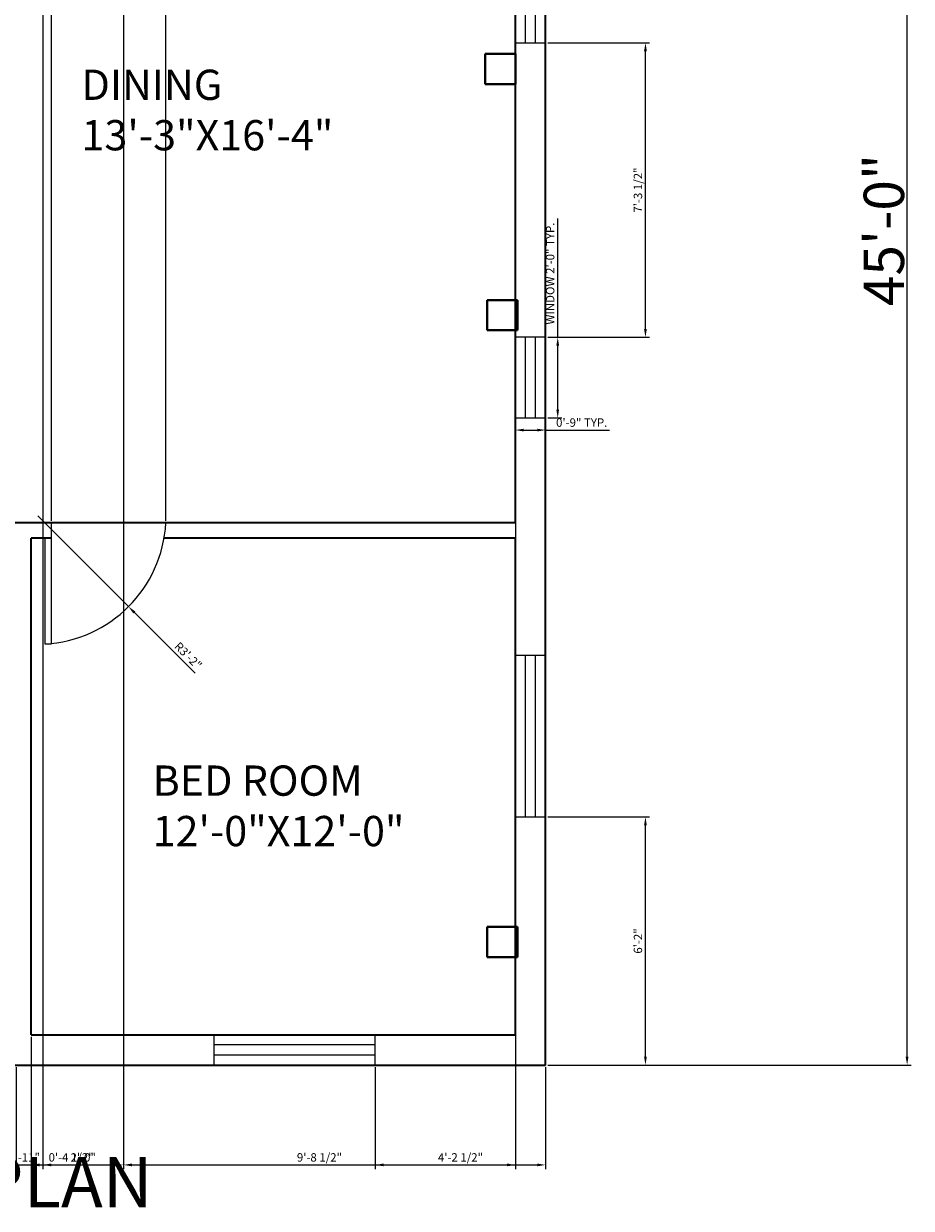
# Model space of a CAD drawing. Units: millimetres. Extents: x 2124 to 2653, y 1244 to 1836.
# Tile 2 of 4: x 2389 to 2653, y 1244 to 1597. Entities that reach past the tile are written whole.
import ezdxf

# ---------------------------------------------------------------- set-up
doc = ezdxf.new("R2010")
doc.units = ezdxf.units.MM
for name, color, linetype, lineweight in [('A-ANNO-DIMS', 2, 'Continuous', 18), ('A-ANNO-TITL', 7, 'Continuous', 35), ('A-AREA-IDEN', 7, 'Continuous', 18), ('A-COLS', 1, 'Continuous', 40), ('A-DOOR', 3, 'Continuous', 18), ('A-GLAZ', 4, 'Continuous', 18), ('A-WALL', 7, 'Continuous', 35)]:
    doc.layers.add(name, color=color, linetype=linetype, lineweight=lineweight)
doc.styles.get("Standard").update_dxf_attribs({"font": 'arial.ttf'})
doc.dimstyles.new('ISO-25', dxfattribs={"dimtxt": 2.5, "dimasz": 2.5, "dimexe": 1.25, "dimexo": 0.625, "dimtad": 1, "dimdec": 0, "dimlunit": 3, "dimtxsty": 'Standard', "dimcen": 2.5, "dimadec": 0, "dimazin": 0, "dimtfac": 1, "dimtdec": 0, "dimtmove": 0, "dimatfit": 3, "dimfxl": 1, "dimarcsym": 0})

# ---------------------------------------------------------------- blocks, each defined once
blk = doc.blocks.new('*D9')
at = {"layer": 'A-ANNO-DIMS', "color": 0, "lineweight": -2, "transparency": 16777216}
for p, q in [((2544.38, 1783.74), (2652.54, 1783.74)), ((2651.29, 1289.47), (2651.29, 1781.24)), ((2544.38, 1286.97), (2652.54, 1286.97))]:
    blk.add_line(p, q, dxfattribs=at)
at = {"layer": 'A-ANNO-DIMS', "color": 0, "transparency": 16777216}
for points in [[(2650.87, 1781.24), (2651.71, 1781.24), (2651.29, 1783.74)], [(2650.87, 1289.47), (2651.71, 1289.47), (2651.29, 1286.97)]]:
    blk.add_solid(points, dxfattribs=at)
at = {"layer": 'Defpoints', "color": 0, "transparency": 16777216}
for p in [(2543.76, 1783.74), (2651.29, 1783.74), (2543.76, 1286.97)]:
    blk.add_point(p, dxfattribs=at)
at = {"layer": 'A-ANNO-DIMS', "color": 0, "transparency": 16777216, "insert": (2644.38, 1535.36), "char_height": 2.5, "width": 21.1968, "attachment_point": 5, "rotation": 90}
blk.add_mtext('{\\fCambria|b0|i0|c0|p18;\\H4.8x;45\'-0"}', dxfattribs=at)
blk = doc.blocks.new('WINDOW-4FT')
for p, q in [((48, 9), (0, 9)), ((0, 9), (0, 0)), ((48, 0), (48, 9)), ((48, 6), (0, 6)), ((48, 3), (0, 3)), ((0, 0), (48, 0))]:
    blk.add_line(p, q)
blk = doc.blocks.new('WINDOW-2FT')
for p, q in [((9, 24), (0, 24)), ((0, 24), (0, 0)), ((3, 0), (3, 24)), ((6, 0), (6, 24)), ((9, 0), (9, 24)), ((0, 0), (9, 0))]:
    blk.add_line(p, q)
blk = doc.blocks.new('COLUMN-9IN-SQ')
for p, q in [((9, 9), (0, 9)), ((0, 9), (0, 0)), ((9, 0), (9, 9)), ((0, 0), (9, 0))]:
    blk.add_line(p, q)
blk = doc.blocks.new('*D18')
at = {"layer": 'A-ANNO-DIMS', "color": 0, "lineweight": -2, "transparency": 16777216}
for p, q in [((2547.36, 1503.47), (2547.36, 1538.85)), ((2544.38, 1503.47), (2548.61, 1503.47)), ((2547.36, 1481.97), (2547.36, 1500.97)), ((2544.38, 1479.47), (2548.61, 1479.47))]:
    blk.add_line(p, q, dxfattribs=at)
at = {"layer": 'A-ANNO-DIMS', "color": 0, "transparency": 16777216}
for points in [[(2546.94, 1500.97), (2547.77, 1500.97), (2547.36, 1503.47)], [(2546.94, 1481.97), (2547.77, 1481.97), (2547.36, 1479.47)]]:
    blk.add_solid(points, dxfattribs=at)
at = {"layer": 'Defpoints', "color": 0, "transparency": 16777216}
for p in [(2543.76, 1503.47), (2547.36, 1503.47), (2543.76, 1479.47)]:
    blk.add_point(p, dxfattribs=at)
at = {"layer": 'A-ANNO-DIMS', "color": 0, "transparency": 16777216, "insert": (2545.44, 1522.41), "char_height": 2.5, "attachment_point": 5, "rotation": 90}
blk.add_mtext('WINDOW 2\'-0" TYP.', dxfattribs=at)
blk = doc.blocks.new('*D19')
at = {"layer": 'A-ANNO-DIMS', "color": 0, "lineweight": -2, "transparency": 16777216}
for p, q in [((2534.76, 1478.84), (2534.76, 1474.62)), ((2543.76, 1478.84), (2543.76, 1474.62)), ((2537.26, 1475.87), (2541.26, 1475.87)), ((2543.76, 1475.87), (2562.75, 1475.87))]:
    blk.add_line(p, q, dxfattribs=at)
at = {"layer": 'A-ANNO-DIMS', "color": 0, "transparency": 16777216}
for points in [[(2537.26, 1476.28), (2537.26, 1475.45), (2534.76, 1475.87)], [(2541.26, 1476.28), (2541.26, 1475.45), (2543.76, 1475.87)]]:
    blk.add_solid(points, dxfattribs=at)
at = {"layer": 'Defpoints', "color": 0, "transparency": 16777216}
for p in [(2534.76, 1479.47), (2543.76, 1479.47), (2543.76, 1475.87)]:
    blk.add_point(p, dxfattribs=at)
at = {"layer": 'A-ANNO-DIMS', "color": 0, "transparency": 16777216, "insert": (2554.5, 1477.77), "char_height": 2.5, "attachment_point": 5}
blk.add_mtext('0\'-9" TYP.', dxfattribs=at)
blk = doc.blocks.new('*D23')
at = {"layer": 'A-ANNO-DIMS', "color": 0, "lineweight": -2, "transparency": 16777216}
for p, q in [((2493.1, 1286.35), (2493.1, 1256.02)), ((2543.76, 1286.35), (2543.76, 1256.02)), ((2495.6, 1257.27), (2541.26, 1257.27))]:
    blk.add_line(p, q, dxfattribs=at)
at = {"layer": 'A-ANNO-DIMS', "color": 0, "transparency": 16777216}
for points in [[(2495.6, 1257.69), (2495.6, 1256.86), (2493.1, 1257.27)], [(2541.26, 1257.69), (2541.26, 1256.86), (2543.76, 1257.27)]]:
    blk.add_solid(points, dxfattribs=at)
at = {"layer": 'Defpoints', "color": 0, "transparency": 16777216}
for p in [(2493.1, 1286.97), (2543.76, 1286.97), (2543.76, 1257.27)]:
    blk.add_point(p, dxfattribs=at)
at = {"layer": 'A-ANNO-DIMS', "color": 0, "transparency": 16777216, "insert": (2518.43, 1259.19), "char_height": 2.5, "attachment_point": 5}
blk.add_mtext('4\'-2 1/2"', dxfattribs=at)
blk = doc.blocks.new('*D26')
at = {"layer": 'A-ANNO-DIMS', "color": 0, "lineweight": -2, "transparency": 16777216}
for p, q in [((2544.38, 1591.07), (2574.71, 1591.07)), ((2573.46, 1505.97), (2573.46, 1588.57)), ((2544.38, 1503.47), (2574.71, 1503.47))]:
    blk.add_line(p, q, dxfattribs=at)
at = {"layer": 'A-ANNO-DIMS', "color": 0, "transparency": 16777216}
for points in [[(2573.04, 1588.57), (2573.87, 1588.57), (2573.46, 1591.07)], [(2573.04, 1505.97), (2573.87, 1505.97), (2573.46, 1503.47)]]:
    blk.add_solid(points, dxfattribs=at)
at = {"layer": 'Defpoints', "color": 0, "transparency": 16777216}
for p in [(2543.76, 1591.07), (2573.46, 1591.07), (2543.76, 1503.47)]:
    blk.add_point(p, dxfattribs=at)
at = {"layer": 'A-ANNO-DIMS', "color": 0, "transparency": 16777216, "insert": (2571.54, 1547.27), "char_height": 2.5, "attachment_point": 5, "rotation": 90}
blk.add_mtext('7\'-3 1/2"', dxfattribs=at)
blk = doc.blocks.new('*D27')
at = {"layer": 'A-ANNO-DIMS', "color": 0, "lineweight": -2, "transparency": 16777216}
for p, q in [((2544.38, 1360.81), (2574.71, 1360.81)), ((2573.46, 1289.47), (2573.46, 1358.31)), ((2544.38, 1286.97), (2574.71, 1286.97))]:
    blk.add_line(p, q, dxfattribs=at)
at = {"layer": 'A-ANNO-DIMS', "color": 0, "transparency": 16777216}
for points in [[(2573.04, 1358.31), (2573.87, 1358.31), (2573.46, 1360.81)], [(2573.04, 1289.47), (2573.87, 1289.47), (2573.46, 1286.97)]]:
    blk.add_solid(points, dxfattribs=at)
at = {"layer": 'Defpoints', "color": 0, "transparency": 16777216}
for p in [(2543.76, 1360.81), (2573.46, 1360.81), (2543.76, 1286.97)]:
    blk.add_point(p, dxfattribs=at)
at = {"layer": 'A-ANNO-DIMS', "color": 0, "transparency": 16777216, "insert": (2571.55, 1323.89), "char_height": 2.5, "attachment_point": 5, "rotation": 90}
blk.add_mtext('6\'-2"', dxfattribs=at)
blk = doc.blocks.new('*D43')
at = {"layer": 'A-ANNO-DIMS', "color": 0, "lineweight": -2, "transparency": 16777216}
for p, q in [((2383.02, 1645.62), (2383.02, 1256.02)), ((2394.21, 1645.62), (2394.21, 1256.02)), ((2385.52, 1257.27), (2391.71, 1257.27))]:
    blk.add_line(p, q, dxfattribs=at)
at = {"layer": 'A-ANNO-DIMS', "color": 0, "transparency": 16777216}
for points in [[(2385.52, 1257.69), (2385.52, 1256.86), (2383.02, 1257.27)], [(2391.71, 1257.69), (2391.71, 1256.86), (2394.21, 1257.27)]]:
    blk.add_solid(points, dxfattribs=at)
at = {"layer": 'Defpoints', "color": 0, "transparency": 16777216}
for p in [(2383.02, 1646.24), (2394.21, 1646.24), (2394.21, 1257.27)]:
    blk.add_point(p, dxfattribs=at)
at = {"layer": 'A-ANNO-DIMS', "color": 0, "transparency": 16777216, "insert": (2388.62, 1259.18), "char_height": 2.5, "attachment_point": 5}
blk.add_mtext('0\'-11"', dxfattribs=at)
blk = doc.blocks.new('*D44')
at = {"layer": 'A-ANNO-DIMS', "color": 0, "lineweight": -2, "transparency": 16777216}
for p, q in [((2394.21, 1645.62), (2394.21, 1256.02)), ((2418.21, 1645.62), (2418.21, 1256.02)), ((2396.71, 1257.27), (2415.71, 1257.27))]:
    blk.add_line(p, q, dxfattribs=at)
at = {"layer": 'A-ANNO-DIMS', "color": 0, "transparency": 16777216}
for points in [[(2396.71, 1257.69), (2396.71, 1256.86), (2394.21, 1257.27)], [(2415.71, 1257.69), (2415.71, 1256.86), (2418.21, 1257.27)]]:
    blk.add_solid(points, dxfattribs=at)
at = {"layer": 'Defpoints', "color": 0, "transparency": 16777216}
for p in [(2394.21, 1646.24), (2418.21, 1646.24), (2418.21, 1257.27)]:
    blk.add_point(p, dxfattribs=at)
at = {"layer": 'A-ANNO-DIMS', "color": 0, "transparency": 16777216, "insert": (2406.21, 1259.18), "char_height": 2.5, "attachment_point": 5}
blk.add_mtext('2\'-0"', dxfattribs=at)
blk = doc.blocks.new('*D45')
at = {"layer": 'A-ANNO-DIMS', "color": 0, "lineweight": -2, "transparency": 16777216}
for p, q in [((2418.21, 1645.62), (2418.21, 1256.02)), ((2534.76, 1645.62), (2534.76, 1256.02)), ((2420.71, 1257.27), (2532.26, 1257.27))]:
    blk.add_line(p, q, dxfattribs=at)
at = {"layer": 'A-ANNO-DIMS', "color": 0, "transparency": 16777216}
for points in [[(2420.71, 1257.69), (2420.71, 1256.86), (2418.21, 1257.27)], [(2532.26, 1257.69), (2532.26, 1256.86), (2534.76, 1257.27)]]:
    blk.add_solid(points, dxfattribs=at)
at = {"layer": 'Defpoints', "color": 0, "transparency": 16777216}
for p in [(2418.21, 1646.24), (2534.76, 1646.24), (2534.76, 1257.27)]:
    blk.add_point(p, dxfattribs=at)
at = {"layer": 'A-ANNO-DIMS', "color": 0, "transparency": 16777216, "insert": (2476.48, 1259.19), "char_height": 2.5, "attachment_point": 5}
blk.add_mtext('9\'-8 1/2"', dxfattribs=at)
blk = doc.blocks.new('*D47')
at = {"layer": 'A-ANNO-DIMS', "color": 0, "lineweight": -2, "transparency": 16777216}
for p, q in [((2365.24, 1448.87), (2365.24, 1814.69)), ((2367.74, 1813.44), (2394.29, 1813.44)), ((2396.79, 1448.87), (2396.79, 1814.69))]:
    blk.add_line(p, q, dxfattribs=at)
at = {"layer": 'A-ANNO-DIMS', "color": 0, "transparency": 16777216}
for points in [[(2367.74, 1813.86), (2367.74, 1813.02), (2365.24, 1813.44)], [(2394.29, 1813.86), (2394.29, 1813.02), (2396.79, 1813.44)]]:
    blk.add_solid(points, dxfattribs=at)
at = {"layer": 'Defpoints', "color": 0, "transparency": 16777216}
for p in [(2396.79, 1813.44), (2365.24, 1448.24), (2396.79, 1448.24)]:
    blk.add_point(p, dxfattribs=at)
at = {"layer": 'A-ANNO-DIMS', "color": 0, "transparency": 16777216, "insert": (2381.02, 1815.36), "char_height": 2.5, "attachment_point": 5}
blk.add_mtext('2\'-7 1/2"', dxfattribs=at)
blk = doc.blocks.new('*D48')
at = {"layer": 'A-ANNO-DIMS', "color": 0, "lineweight": -2, "transparency": 16777216}
for p, q in [((2396.79, 1448.87), (2396.79, 1814.69)), ((2399.29, 1813.44), (2428.29, 1813.44)), ((2430.79, 1448.87), (2430.79, 1814.69))]:
    blk.add_line(p, q, dxfattribs=at)
at = {"layer": 'A-ANNO-DIMS', "color": 0, "transparency": 16777216}
for points in [[(2399.29, 1813.86), (2399.29, 1813.02), (2396.79, 1813.44)], [(2428.29, 1813.86), (2428.29, 1813.02), (2430.79, 1813.44)]]:
    blk.add_solid(points, dxfattribs=at)
at = {"layer": 'Defpoints', "color": 0, "transparency": 16777216}
for p in [(2430.79, 1813.44), (2396.79, 1448.24), (2430.79, 1448.24)]:
    blk.add_point(p, dxfattribs=at)
at = {"layer": 'A-ANNO-DIMS', "color": 0, "transparency": 16777216, "insert": (2413.79, 1815.34), "char_height": 2.5, "attachment_point": 5}
blk.add_mtext('2\'-10"', dxfattribs=at)
blk = doc.blocks.new('*D49')
at = {"layer": 'A-ANNO-DIMS', "color": 0, "lineweight": -2, "transparency": 16777216}
for p, q in [((2430.79, 1448.87), (2430.79, 1814.69)), ((2433.29, 1813.44), (2532.26, 1813.44)), ((2534.76, 1448.87), (2534.76, 1814.69))]:
    blk.add_line(p, q, dxfattribs=at)
at = {"layer": 'A-ANNO-DIMS', "color": 0, "transparency": 16777216}
for points in [[(2433.29, 1813.86), (2433.29, 1813.02), (2430.79, 1813.44)], [(2532.26, 1813.86), (2532.26, 1813.02), (2534.76, 1813.44)]]:
    blk.add_solid(points, dxfattribs=at)
at = {"layer": 'Defpoints', "color": 0, "transparency": 16777216}
for p in [(2534.76, 1813.44), (2430.79, 1448.24), (2534.76, 1448.24)]:
    blk.add_point(p, dxfattribs=at)
at = {"layer": 'A-ANNO-DIMS', "color": 0, "transparency": 16777216, "insert": (2482.77, 1815.34), "char_height": 2.5, "attachment_point": 5}
blk.add_mtext('8\'-8"', dxfattribs=at)
blk = doc.blocks.new('*D52')
at = {"layer": 'A-ANNO-DIMS', "color": 0, "lineweight": -2, "transparency": 16777216}
for p, q in [((2390.76, 1295.35), (2390.76, 1256.02)), ((2386.26, 1286.35), (2386.26, 1256.02)), ((2383.76, 1257.27), (2381.26, 1257.27)), ((2386.26, 1257.27), (2390.76, 1257.27)), ((2393.26, 1257.27), (2409.48, 1257.27))]:
    blk.add_line(p, q, dxfattribs=at)
at = {"layer": 'A-ANNO-DIMS', "color": 0, "transparency": 16777216}
for points in [[(2383.76, 1257.69), (2383.76, 1256.86), (2386.26, 1257.27)], [(2393.26, 1257.69), (2393.26, 1256.86), (2390.76, 1257.27)]]:
    blk.add_solid(points, dxfattribs=at)
at = {"layer": 'Defpoints', "color": 0, "transparency": 16777216}
for p in [(2390.76, 1295.97), (2386.26, 1286.97), (2390.76, 1257.27)]:
    blk.add_point(p, dxfattribs=at)
at = {"layer": 'A-ANNO-DIMS', "color": 0, "transparency": 16777216, "insert": (2402.62, 1259.19), "char_height": 2.5, "attachment_point": 5}
blk.add_mtext('0\'-4 1/2"', dxfattribs=at)
blk = doc.blocks.new('*D54')
at = {"layer": 'A-ANNO-DIMS', "color": 0, "lineweight": -2, "transparency": 16777216}
for p, q in [((2392.72, 1450.31), (2419.68, 1423.35)), ((2439.49, 1403.54), (2421.45, 1421.58))]:
    blk.add_line(p, q, dxfattribs=at)
at = {"layer": 'A-ANNO-DIMS', "color": 0, "transparency": 16777216}
blk.add_solid([(2421.74, 1421.88), (2421.15, 1421.29), (2419.68, 1423.35)], dxfattribs=at)
at = {"layer": 'Defpoints', "color": 0, "transparency": 16777216}
for p in [(2392.72, 1450.31), (2419.68, 1423.35)]:
    blk.add_point(p, dxfattribs=at)
at = {"layer": 'A-ANNO-DIMS', "color": 0, "transparency": 16777216, "insert": (2437.2, 1408.52), "char_height": 2.5, "attachment_point": 5, "rotation": 314.9995}
blk.add_mtext('R3\'-2"', dxfattribs=at)

msp = doc.modelspace()

# ---------------------------------------------------------------- linework, layer by layer
at = {"layer": 'A-DOOR'}
for p, q in [((2430.79, 1448.24), (2394.79, 1448.24)), ((2396.79, 1412.24), (2396.79, 1448.24)), ((2394.79, 1443.74), (2394.79, 1412.24)), ((2394.79, 1412.24), (2396.79, 1412.24))]:
    msp.add_line(p, q, dxfattribs=at)
msp.add_arc((2392.72, 1450.31), 38.13, 273.1129, 356.8871, dxfattribs=at)
at = {"layer": 'A-WALL'}
for p, q in [((2543.76, 1286.97), (2543.76, 1783.74)), ((2534.76, 1448.24), (2534.76, 1646.24)), ((2534.76, 1448.24), (2301.76, 1448.24)), ((2390.76, 1295.97), (2390.76, 1443.74)), ((2396.79, 1443.74), (2390.76, 1443.74)), ((2534.76, 1443.74), (2430.28, 1443.74)), ((2534.76, 1295.97), (2534.76, 1443.74)), ((2390.76, 1295.97), (2534.76, 1295.97)), ((2159.76, 1286.97), (2543.76, 1286.97))]:
    msp.add_line(p, q, dxfattribs=at)

# ---------------------------------------------------------------- block references
at = {"layer": 'A-COLS'}
for p in [(2525.76, 1578.8), (2526.38, 1505.54), (2526.38, 1319.05)]:
    msp.add_blockref('COLUMN-9IN-SQ', p, dxfattribs=at)
at = {"layer": 'A-GLAZ'}
for name, p in [('WINDOW-2FT', (2534.76, 1591.07)), ('WINDOW-2FT', (2534.76, 1479.47)), ('WINDOW-4FT', (2445.1, 1286.97))]:
    msp.add_blockref(name, p, dxfattribs=at)
at = {"layer": 'A-GLAZ', "rotation": 270.0000000000006}
msp.add_blockref('WINDOW-4FT', (2534.76, 1408.81), dxfattribs=at)

# ---------------------------------------------------------------- texts
at = {"layer": 'A-ANNO-TITL', "insert": (2260.19, 1259.63), "char_height": 15, "attachment_point": 1}
msp.add_mtext_dynamic_manual_height_columns('{\\fCambria|b0|i0|c0|p18;1 ST FLOOR PLAN}', width=375.7159, gutter_width=12.5, heights=[0], dxfattribs=at)
at = {"layer": 'A-AREA-IDEN', "char_height": 9, "attachment_point": 1}
for s, width, insert in [('{\\fCambria|b0|i0|c0|p18;DINING\\P13\'-3"X16\'-4"}', 106.8393, (2405.71, 1583.08)), ('{\\fCambria|b0|i0|c0|p18;BED ROOM\\P12\'-0"X12\'-0"}', 93.0425, (2426.87, 1376.09))]:
    msp.add_mtext_dynamic_manual_height_columns(s, width=width, gutter_width=12.5, heights=[0], dxfattribs=dict(at, insert=insert))

# ---------------------------------------------------------------- dimensions: what is measured, and where the dimension line sits
at = {"layer": 'A-ANNO-DIMS'}
for base, p1, p2, picture, middle in [((2396.7929, 1813.4406), (2365.2427, 1448.2406), (2396.7929, 1448.2406), '*D47', (2381.0178, 1815.3582)), ((2430.79, 1813.44), (2396.79, 1448.24), (2430.79, 1448.24), '*D48', (2413.79, 1815.34)), ((2534.76, 1813.44), (2430.79, 1448.24), (2534.76, 1448.24), '*D49', (2482.77, 1815.34)), ((2394.21, 1257.27), (2383.02, 1646.24), (2394.21, 1646.24), '*D43', (2388.62, 1259.18)), ((2418.21, 1257.27), (2394.21, 1646.24), (2418.21, 1646.24), '*D44', (2406.21, 1259.18)), ((2534.7564, 1257.2741), (2418.2124, 1646.2406), (2534.7564, 1646.2406), '*D45', (2476.4844, 1259.1917)), ((2390.76, 1257.27), (2386.26, 1286.97), (2390.76, 1295.97), '*D52', (2402.62, 1259.19)), ((2543.76, 1257.27), (2493.1, 1286.97), (2543.76, 1286.97), '*D23', (2518.43, 1259.19))]:
    dim = msp.add_linear_dim(base=base, p1=p1, p2=p2, dimstyle='ISO-25', override={"dimdec": 1, "dimlfac": 1, "dimrnd": 0, "dimzin": 1, "dimdsep": 46, "dimlunit": 4, "dimfrac": 2}, dxfattribs=at)
    dim.commit()
    dim.dimension.update_dxf_attribs({"geometry": picture, "text_midpoint": middle})
for base, p1, p2, text, override, picture, middle in [((2651.29, 1783.74), (2543.76, 1286.97), (2543.76, 1783.74), '{\\fCambria|b0|i0|c0|p18;\\H4.8x;45\'-0"}', {"dimclrd": 0, "dimclre": 0, "dimclrt": 0}, '*D9', (2644.38, 1535.36)), ((2547.36, 1503.47), (2543.76, 1479.47), (2543.76, 1503.47), 'WINDOW <> TYP.', {"dimdec": 1, "dimlfac": 1, "dimrnd": 0, "dimzin": 1, "dimdsep": 46, "dimlunit": 4, "dimfrac": 2}, '*D18', (2545.44, 1522.41))]:
    dim = msp.add_linear_dim(base=base, p1=p1, p2=p2, angle=90, text=text, dimstyle='ISO-25', override=override, dxfattribs=at)
    dim.commit()
    dim.dimension.update_dxf_attribs({"geometry": picture, "text_midpoint": middle})
for base, p1, p2, picture, middle in [((2573.46, 1591.07), (2543.76, 1503.47), (2543.76, 1591.07), '*D26', (2571.54, 1547.27)), ((2573.46, 1360.81), (2543.76, 1286.97), (2543.76, 1360.81), '*D27', (2571.55, 1323.89))]:
    dim = msp.add_linear_dim(base=base, p1=p1, p2=p2, angle=90, dimstyle='ISO-25', override={"dimdec": 1, "dimlfac": 1, "dimrnd": 0, "dimzin": 1, "dimdsep": 46, "dimlunit": 4, "dimfrac": 2}, dxfattribs=at)
    dim.commit()
    dim.dimension.update_dxf_attribs({"geometry": picture, "text_midpoint": middle})
dim = msp.add_linear_dim(base=(2543.76, 1475.87), p1=(2534.76, 1479.47), p2=(2543.76, 1479.47), text='<> TYP.', dimstyle='ISO-25', override={"dimdec": 1, "dimlfac": 1, "dimrnd": 0, "dimzin": 1, "dimdsep": 46, "dimlunit": 4, "dimfrac": 2}, dxfattribs=at)
dim.commit()
dim.dimension.update_dxf_attribs({"geometry": '*D19', "text_midpoint": (2554.5, 1477.77)})
dim = msp.add_radius_dim(center=(2392.72, 1450.31), mpoint=(2419.68, 1423.35), dimstyle='ISO-25', override={"dimdec": 1, "dimlfac": 1, "dimrnd": 0, "dimzin": 1, "dimdsep": 46, "dimlunit": 4, "dimfrac": 2}, dxfattribs=at)
dim.commit()
dim.dimension.update_dxf_attribs({"geometry": '*D54', "text_midpoint": (2435.86, 1407.18), "dimtype": 164})

doc.saveas('drawing.dxf')
